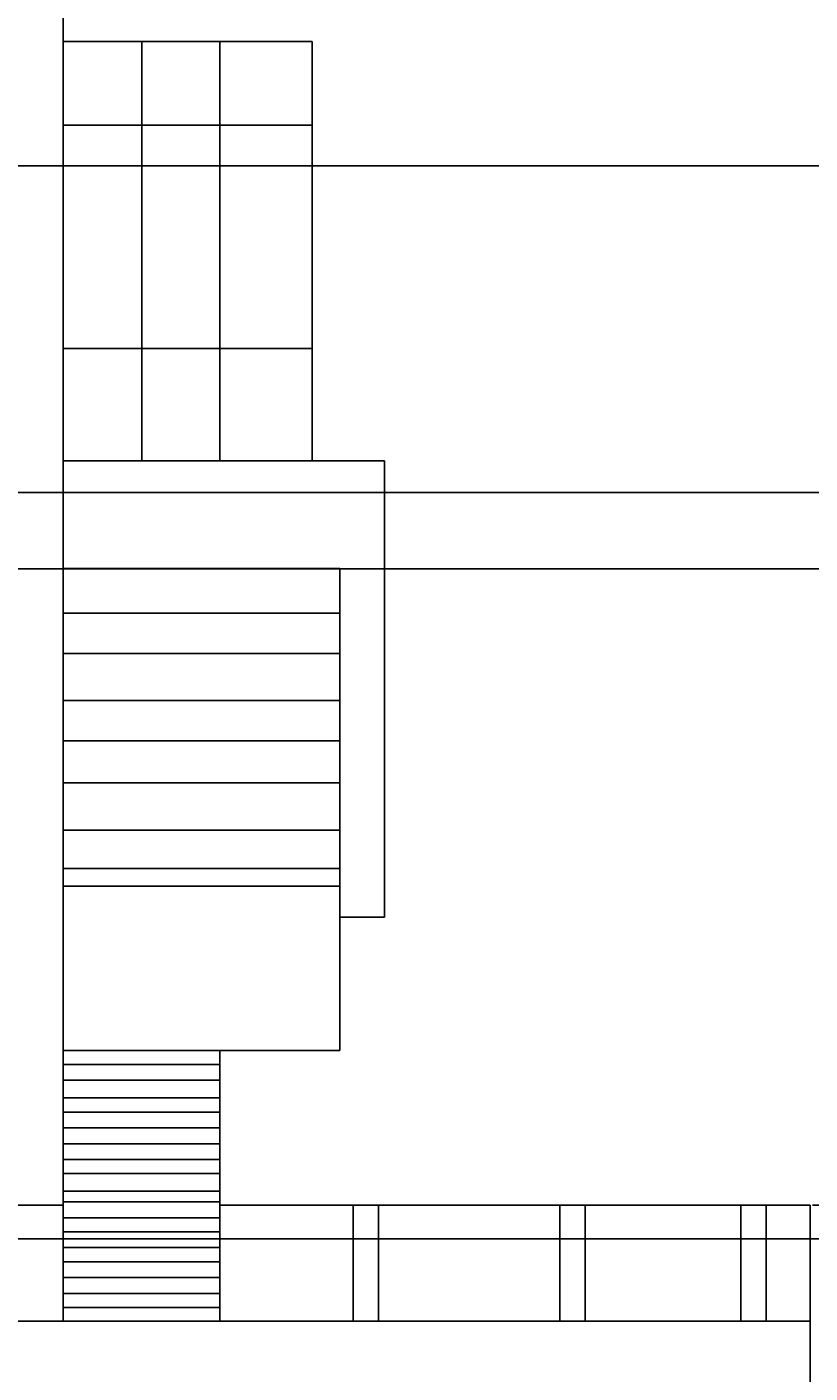
# Model space of a CAD drawing. Units: inches. Extents: x -117 to 121, y -77 to 40.
# Tile 40 of 45: x 72 to 91, y -43 to -10. Entities that reach past the tile are written whole.
import ezdxf

# ---------------------------------------------------------------- set-up
doc = ezdxf.new("R2010")
doc.units = ezdxf.units.IN
doc.header["$MEASUREMENT"] = 0
doc.layers.add('A-ANNO-DIMS', color=2, linetype='Continuous', lineweight=18)
doc.layers.add('A-ELEV', color=7, linetype='Continuous', lineweight=25)
doc.styles.get("Standard").update_dxf_attribs({"font": 'arial.ttf'})
doc.dimstyles.get("Standard").update_dxf_attribs({"dimtxt": 0.18, "dimasz": 0.18, "dimexe": 0.18, "dimexo": 0.0625, "dimgap": 0.09, "dimtad": 0, "dimtih": 1, "dimtoh": 1, "dimdec": 4, "dimzin": 0, "dimdsep": 46, "dimtxsty": 'Standard', "dimcen": 0.09, "dimadec": 0, "dimazin": 0, "dimtfac": 1, "dimtdec": 4, "dimtofl": 0, "dimtmove": 0, "dimatfit": 3, "dimfxl": 1, "dimtolj": 1, "dimtzin": 0, "dimarcsym": 0})

# ---------------------------------------------------------------- blocks, each defined once
blk = doc.blocks.new('*D15')
at = {"layer": 'A-ANNO-DIMS', "color": 0, "lineweight": -2, "transparency": 16777216}
for p, q in [((87.304, -2.653), (120.84, -2.653)), ((120.66, -2.833), (120.66, -20.595)), ((120.66, -38.722), (120.66, -20.959)), ((90.611, -38.902), (120.84, -38.902))]:
    blk.add_line(p, q, dxfattribs=at)
at = {"layer": 'A-ANNO-DIMS', "color": 0, "transparency": 16777216}
for points in [[(120.63, -2.833), (120.69, -2.833), (120.66, -2.653)], [(120.63, -38.722), (120.69, -38.722), (120.66, -38.902)]]:
    blk.add_solid(points, dxfattribs=at)
at = {"layer": 'Defpoints', "color": 0, "transparency": 16777216}
for p in [(87.242, -2.653), (90.549, -38.902), (120.66, -38.902)]:
    blk.add_point(p, dxfattribs=at)
at = {"layer": 'A-ANNO-DIMS', "color": 0, "transparency": 16777216, "insert": (120.66, -20.777), "char_height": 0.18, "attachment_point": 5}
blk.add_mtext('\\A1;36.25', dxfattribs=at)
blk = doc.blocks.new('*D24')
at = {"layer": 'A-ANNO-DIMS', "color": 0, "lineweight": -2, "transparency": 16777216}
for p, q in [((87.242, 3.166), (87.242, 38.61)), ((109.85, -61.313), (109.85, 38.61)), ((87.422, 38.43), (98.081, 38.43)), ((109.67, 38.43), (99.011, 38.43))]:
    blk.add_line(p, q, dxfattribs=at)
at = {"layer": 'A-ANNO-DIMS', "color": 0, "transparency": 16777216}
for points in [[(87.422, 38.46), (87.422, 38.4), (87.242, 38.43)], [(109.67, 38.46), (109.67, 38.4), (109.85, 38.43)]]:
    blk.add_solid(points, dxfattribs=at)
at = {"layer": 'Defpoints', "color": 0, "transparency": 16777216}
for p in [(109.85, 38.43), (87.242, 3.104), (109.85, -61.376)]:
    blk.add_point(p, dxfattribs=at)
at = {"layer": 'A-ANNO-DIMS', "color": 0, "transparency": 16777216, "insert": (98.546, 38.43), "char_height": 0.18, "attachment_point": 5}
blk.add_mtext('\\A1;22.609', dxfattribs=at)
blk = doc.blocks.new('*D49')
at = {"layer": 'A-ANNO-DIMS', "color": 0, "lineweight": -2, "transparency": 16777216}
for p, q in [((-45.422, -23.501), (120.84, -23.501)), ((120.66, -23.681), (120.66, -31.426)), ((120.66, -39.536), (120.66, -31.79)), ((-45.471, -39.716), (120.84, -39.716))]:
    blk.add_line(p, q, dxfattribs=at)
at = {"layer": 'A-ANNO-DIMS', "color": 0, "transparency": 16777216}
for points in [[(120.63, -23.681), (120.69, -23.681), (120.66, -23.501)], [(120.63, -39.536), (120.69, -39.536), (120.66, -39.716)]]:
    blk.add_solid(points, dxfattribs=at)
at = {"layer": 'Defpoints', "color": 0, "transparency": 16777216}
for p in [(-45.485, -23.501), (120.66, -23.501), (-45.533, -39.716)]:
    blk.add_point(p, dxfattribs=at)
at = {"layer": 'A-ANNO-DIMS', "color": 0, "transparency": 16777216, "insert": (120.66, -31.608), "char_height": 0.18, "attachment_point": 5}
blk.add_mtext('\\A1;16.215', dxfattribs=at)
blk = doc.blocks.new('*D50')
at = {"layer": 'A-ANNO-DIMS', "color": 0, "lineweight": -2, "transparency": 16777216}
for p, q in [((-47.458, -13.74), (120.84, -13.74)), ((120.66, -13.92), (120.66, -17.512)), ((120.66, -21.468), (120.66, -17.876)), ((-47.458, -21.648), (120.84, -21.648))]:
    blk.add_line(p, q, dxfattribs=at)
at = {"layer": 'A-ANNO-DIMS', "color": 0, "transparency": 16777216}
for points in [[(120.63, -13.92), (120.69, -13.92), (120.66, -13.74)], [(120.63, -21.468), (120.69, -21.468), (120.66, -21.648)]]:
    blk.add_solid(points, dxfattribs=at)
at = {"layer": 'Defpoints', "color": 0, "transparency": 16777216}
for p in [(-47.521, -13.74), (120.66, -13.74), (-47.521, -21.648)]:
    blk.add_point(p, dxfattribs=at)
at = {"layer": 'A-ANNO-DIMS', "color": 0, "transparency": 16777216, "insert": (120.66, -17.694), "char_height": 0.18, "attachment_point": 5}
blk.add_mtext('\\A1;7.908', dxfattribs=at)

msp = doc.modelspace()

# ---------------------------------------------------------------- linework, layer by layer
at = {"layer": 'A-ELEV'}
for p, q in [((72.4671, -2.6528), (72.4671, -41.7053)), ((78.4905, -10.7374), (72.4671, -10.7374)), ((74.3683, -10.7374), (74.3683, -20.8857)), ((76.2604, -10.7374), (76.2604, -20.8857)), ((78.4905, -10.7374), (78.4905, -20.8857)), ((78.4905, -12.7623), (72.4671, -12.7623)), ((78.4905, -18.162), (72.4671, -18.162)), ((78.4905, -20.8857), (72.4671, -20.8857)), ((78.4905, -20.8857), (80.247, -20.8857)), ((80.247, -20.8857), (80.247, -31.9258)), ((79.1657, -23.4887), (72.4671, -23.4887)), ((79.1657, -31.9258), (79.1657, -23.4887)), ((79.1657, -24.5714), (72.4671, -24.5714)), ((79.1657, -25.545), (72.4671, -25.545)), ((79.1657, -26.688), (72.4671, -26.688)), ((79.1657, -27.6617), (72.4671, -27.6617)), ((79.1657, -28.6777), (72.4671, -28.6777)), ((79.1657, -29.8206), (72.4671, -29.8206)), ((79.1657, -30.752), (72.4671, -30.752)), ((79.1657, -31.1753), (72.4671, -31.1753)), ((80.247, -31.9258), (79.1657, -31.9258)), ((79.1657, -31.9258), (79.1657, -35.1546)), ((79.1657, -35.1546), (72.4671, -35.1546)), ((76.2579, -35.1546), (76.2579, -41.7053)), ((76.2579, -35.4956), (72.4671, -35.4956)), ((76.2579, -35.8791), (72.4671, -35.8791)), ((76.2579, -36.3054), (72.4671, -36.3054)), ((76.2579, -36.6463), (72.4671, -36.6463)), ((76.2579, -37.0299), (72.4671, -37.0299)), ((76.2579, -37.4135), (72.4671, -37.4135)), ((76.2579, -37.7971), (72.4671, -37.7971)), ((76.2579, -38.1381), (72.4671, -38.1381)), ((76.2579, -38.5643), (72.4671, -38.5643)), ((58.4308, -38.9022), (72.4671, -38.9022)), ((76.2579, -38.82), (72.4671, -38.82)), ((76.2579, -38.9022), (90.5486, -38.9022)), ((79.4897, -41.7053), (79.4897, -38.9022)), ((80.1033, -41.7053), (80.1033, -38.9022)), ((84.4867, -41.7053), (84.4867, -38.9022)), ((85.1004, -41.7053), (85.1004, -38.9022)), ((88.8701, -41.7053), (88.8701, -38.9022)), ((89.4838, -41.7053), (89.4838, -38.9022)), ((90.5486, -38.9022), (90.5486, -41.7053)), ((76.2579, -39.2036), (72.4671, -39.2036)), ((76.2579, -39.5446), (72.4671, -39.5446)), ((76.2579, -39.9282), (72.4671, -39.9282)), ((76.2579, -40.2691), (72.4671, -40.2691)), ((76.2579, -40.6527), (72.4671, -40.6527)), ((76.2579, -41.0363), (72.4671, -41.0363)), ((76.2579, -41.3773), (72.4671, -41.3773)), ((72.4671, -41.7053), (68.508, -41.7053)), ((72.4671, -41.7053), (90.5486, -41.7053)), ((90.5486, -44.5456), (90.5486, -41.7053))]:
    msp.add_line(p, q, dxfattribs=at)

# ---------------------------------------------------------------- dimensions: what is measured, and where the dimension line sits
at = {"layer": 'A-ANNO-DIMS'}
dim = msp.add_linear_dim(base=(109.8502, 38.4297), p1=(87.2416, 3.1036), p2=(109.8502, -61.3756), dimstyle='Standard', override={"dimdec": 3, "dimlfac": 1, "dimrnd": 0, "dimzin": 0, "dimdsep": 46, "dimlunit": 2}, dxfattribs=at)
dim.commit()
dim.dimension.update_dxf_attribs({"geometry": '*D24', "text_midpoint": (98.5459, 38.4297)})
for base, p1, p2, override, picture, middle in [((120.6602, -38.9022), (87.2416, -2.6528), (90.5486, -38.9022), {"dimdec": 2, "dimlfac": 1, "dimrnd": 0, "dimzin": 0, "dimdsep": 46, "dimlunit": 2}, '*D15', (120.6602, -20.7775)), ((120.6602, -13.74), (-47.5206, -21.6476), (-47.5206, -13.74), {"dimdec": 3, "dimlfac": 1, "dimrnd": 0, "dimzin": 0, "dimdsep": 46, "dimlunit": 2}, '*D50', (120.6602, -17.6938)), ((120.6602, -23.5007), (-45.5331, -39.716), (-45.4848, -23.5007), {"dimdec": 3, "dimlfac": 1, "dimrnd": 0, "dimzin": 0, "dimdsep": 46, "dimlunit": 2}, '*D49', (120.6602, -31.6083))]:
    dim = msp.add_linear_dim(base=base, p1=p1, p2=p2, angle=90, dimstyle='Standard', override=override, dxfattribs=at)
    dim.commit()
    dim.dimension.update_dxf_attribs({"geometry": picture, "text_midpoint": middle})

doc.saveas('drawing.dxf')
